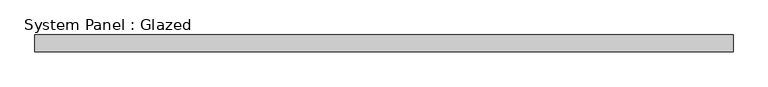
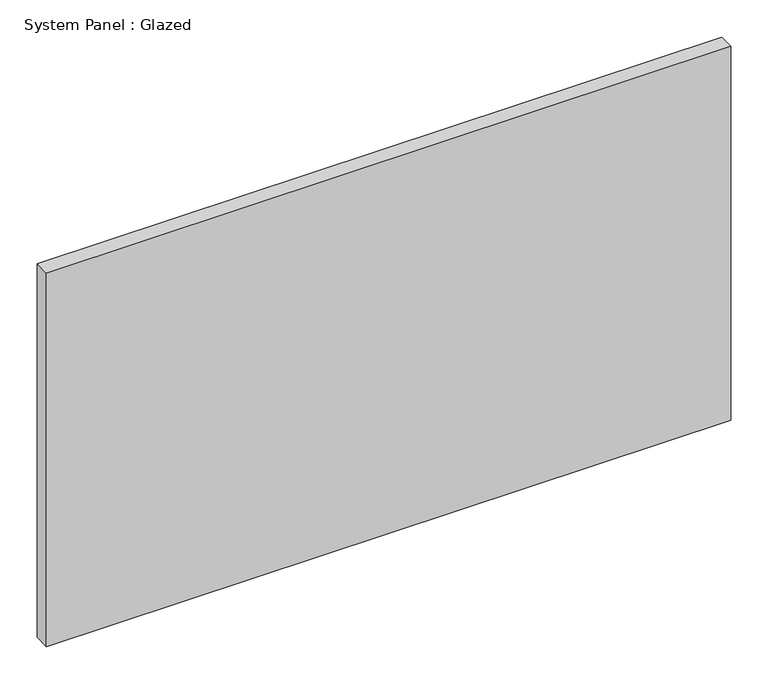
"""IFC4 building model written with IfcOpenShell, lengths in millimetres: plate geometry, System Panel : Glazed."""

from ifc_helpers import new_model, si_unit, origin, origin_with_axes, place, context, project, spatial, polyline, outline, extrude, source, transform, mapped, element, save


def system_panel_glazed_ecc42322(model_context):
    return source(origin(), model_context, "Body", "SweptSolid", [
        extrude(outline(polyline([(533.532314, 19.05), (-533.532314, 19.05), (-533.532314, 44.45), (533.532314, 44.45), (533.532314, 19.05)])), origin_with_axes(), (0.0, 0.0, 1.0), 615.95),
    ])


if __name__ == "__main__":
    model = new_model("IFC4")
    model_context = context("Model", 3, world=origin())
    ifc_project = project(units=[si_unit("LENGTHUNIT", "METRE", prefix="MILLI")], contexts=[model_context])
    site = spatial("IfcSite", under=ifc_project)
    building = spatial("IfcBuilding", under=site)
    placement = place(None, origin())
    system_panel_glazed_shape = system_panel_glazed_ecc42322(model_context)
    element("IfcPlate", 1, ObjectType="System Panel : Glazed", at=placement, inside=building, context=model_context, shape_type="MappedRepresentation", body=[
        mapped(system_panel_glazed_shape, transform((0.0, 0.0, 0.0), x_axis=(1.0, 0.0, 0.0), y_axis=(0.0, 1.0, 0.0), z_axis=(0.0, 0.0, 1.0))),
    ])
    save(model, "model.ifc")

# Revit data of these elements
# Type "System Panel : Glazed"
#   Construction Type Id = "GSP4R"
#   Analytic Construction = "1/8 in Pilkington single glazing"
#   Visual Light Transmittance = 0.9
#   Solar Heat Gain Coefficient = 0.86
#   Heat Transfer Coefficient (U) = 1.18115 BTU/(h·ft²·°F)
#   Define Thermal Properties by = 1
# Element 1 (IfcPlate, "System Panel : Glazed")
#   Materials on its faces: "Glass"
# Materials
#   "Glass": class "Glass", colour RGB 0 128 192, transparency 0.75, Description = "Soda Lime Glass", Cost = 0
